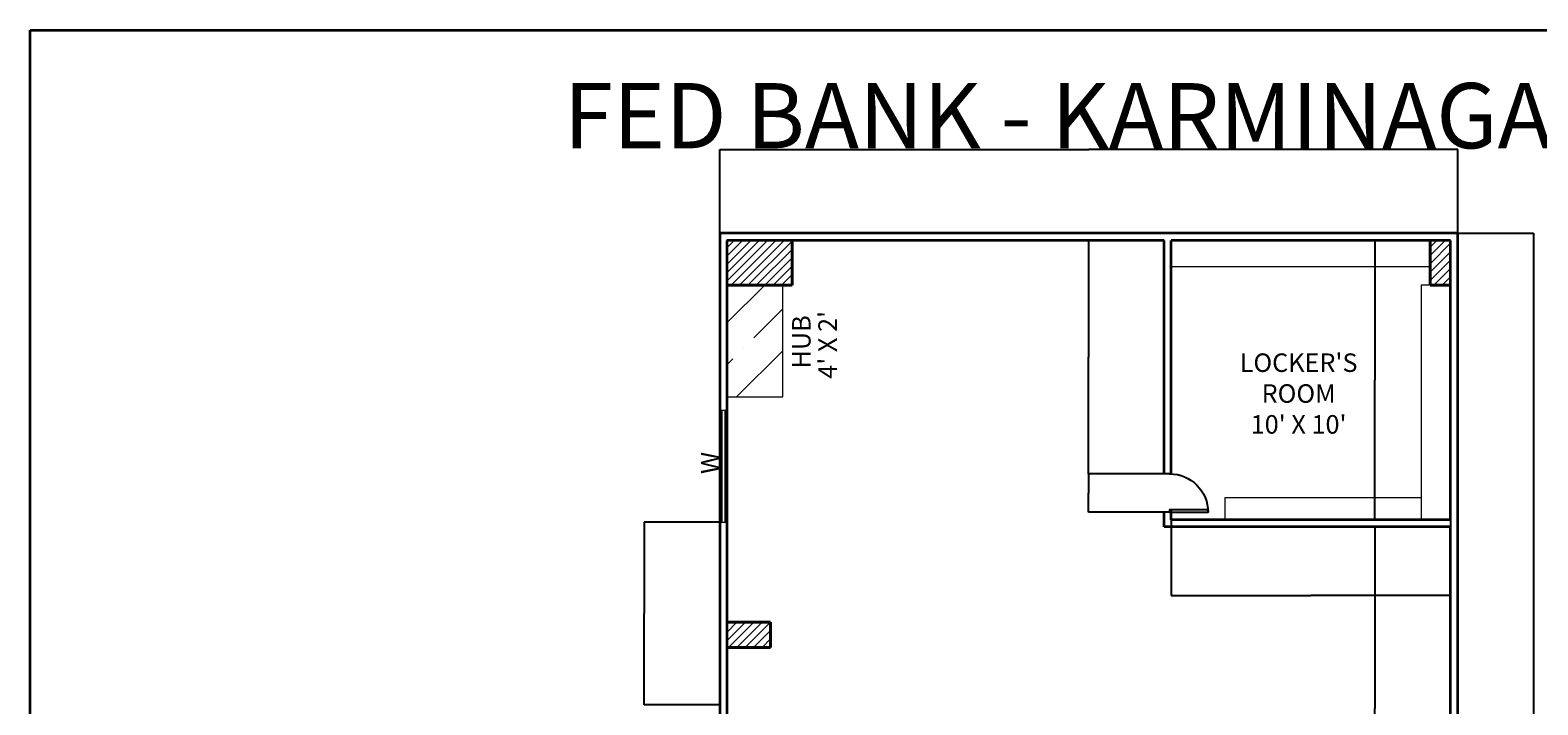
# Model space of a CAD drawing. Units: millimetres. Extents: x -5297 to 19051, y -14478 to 4427.
# Tile 3 of 4: x -5297 to 10888, y -2816 to 4427. Entities that reach past the tile are written whole.
import ezdxf

# ---------------------------------------------------------------- set-up
doc = ezdxf.new("R2010")
doc.units = ezdxf.units.MM
for name, color, linetype, lineweight in [('A-ANNO-DIMS', 2, 'Continuous', 18), ('A-ANNO-TEXT', 7, 'Continuous', 18), ('A-ANNO-TTLB', 7, 'Continuous', 35), ('A-AREA-IDEN', 7, 'Continuous', 25), ('A-COLS', 7, 'Continuous', 40), ('A-COLS-PATT', 252, 'Continuous', 13), ('A-DOOR', 3, 'Continuous', 25), ('A-EQPM', 8, 'Continuous', 20), ('A-EQPM-PATT', 252, 'Continuous', 13), ('A-FLOR-CASE', 9, 'Continuous', 20), ('A-GLAZ', 4, 'Continuous', 18), ('A-WALL', 7, 'Continuous', 35)]:
    doc.layers.add(name, color=color, linetype=linetype, lineweight=lineweight)
doc.styles.get("Standard").update_dxf_attribs({"font": 'arial.ttf'})
doc.dimstyles.get("Standard").update_dxf_attribs({"dimtxt": 0.18, "dimasz": 0.18, "dimexe": 0.18, "dimexo": 0.0625, "dimgap": 0.09, "dimtad": 0, "dimtih": 1, "dimtoh": 1, "dimdec": 4, "dimzin": 0, "dimdsep": 46, "dimtxsty": 'Standard', "dimcen": 0.09, "dimadec": 0, "dimazin": 0, "dimtfac": 1, "dimtdec": 4, "dimtofl": 0, "dimtmove": 0, "dimatfit": 3, "dimfxl": 1, "dimtolj": 1, "dimtzin": 0, "dimarcsym": 0})

# ---------------------------------------------------------------- blocks, each defined once
blk = doc.blocks.new('*U5')
for p, q in [((-700, 0), (-700, 99.99999999999996)), ((0, 0), (0, 99.99999999999999))]:
    blk.add_line(p, q)
blk.add_lwpolyline([(0, 0), (-1.137e-13, -700), (-43.75000000000011, -700), (-43.75, 1.42e-14)], close=True)
blk.add_arc((0, 0), 700, 180, 270)
blk = doc.blocks.new('WIN-1200')
for p, q in [((-4.547e-13, 1200.930645756219), (76.19999999999936, 1200.930645756219)), ((23.09999999999945, 1200.930645756219), (23.09999999999945, 0.9306457562195191)), ((53.09999999999945, 1200.930645756219), (53.09999999999945, 0.9306457562195191)), ((-4.547e-13, 0), (76.19999999999936, 0))]:
    blk.add_line(p, q)
blk = doc.blocks.new('*D20')
at = {"layer": 'A-ANNO-DIMS', "color": 0, "lineweight": -2, "transparency": 16777216}
for p, q in [((2105.501609, 2246.251823), (2105.501609, 3145.869928)), ((2105.681609, 3145.689928), (6066.344494402454, 3145.689928)), ((10027.721609, 3145.689928), (6067.058723597544, 3145.689928)), ((10027.901609, 2246.251823), (10027.901609, 3145.869928))]:
    blk.add_line(p, q, dxfattribs=at)
at = {"layer": 'A-ANNO-DIMS', "color": 0, "transparency": 16777216}
for points in [[(2105.681609, 3145.719928), (2105.681609, 3145.659928), (2105.501609, 3145.689928)], [(10027.721609, 3145.719928), (10027.721609, 3145.659928), (10027.901609, 3145.689928)]]:
    blk.add_solid(points, dxfattribs=at)
at = {"layer": 'Defpoints', "color": 0, "transparency": 16777216}
for p in [(10027.901609, 3145.689928), (2105.501609, 2246.189323), (10027.901609, 2246.189323)]:
    blk.add_point(p, dxfattribs=at)
at = {"layer": 'A-ANNO-DIMS', "color": 0, "transparency": 16777216, "insert": (6066.701608999999, 3145.689928), "char_height": 0.18, "attachment_point": 5}
blk.add_mtext('\\A1;7922', dxfattribs=at)
blk = doc.blocks.new('*D21')
at = {"layer": 'A-ANNO-DIMS', "color": 0, "lineweight": -2, "transparency": 16777216}
for p, q in [((10027.964109, 2246.189323000001), (10840.581609, 2246.189323000001)), ((10840.401609, 2246.009323000001), (10840.401609, -5417.56906597067)), ((10840.40160900001, -13081.511384), (10840.401609, -5417.932995029333)), ((10027.964109, -13081.691384), (10840.58160900001, -13081.691384))]:
    blk.add_line(p, q, dxfattribs=at)
at = {"layer": 'A-ANNO-DIMS', "color": 0, "transparency": 16777216}
for points in [[(10840.371609, 2246.009323000001), (10840.431609, 2246.009323000001), (10840.401609, 2246.189323000001)], [(10840.37160900001, -13081.511384), (10840.43160900001, -13081.511384), (10840.40160900001, -13081.691384)]]:
    blk.add_solid(points, dxfattribs=at)
at = {"layer": 'Defpoints', "color": 0, "transparency": 16777216}
for p in [(10027.901609, 2246.189323000001), (10027.901609, -13081.691384), (10840.40160900001, -13081.691384)]:
    blk.add_point(p, dxfattribs=at)
at = {"layer": 'A-ANNO-DIMS', "color": 0, "transparency": 16777216, "insert": (10840.401609, -5417.751030500004), "char_height": 0.18, "attachment_point": 5}
blk.add_mtext('\\A1;15328', dxfattribs=at)
blk = doc.blocks.new('*D24')
at = {"layer": 'A-ANNO-DIMS', "color": 0, "lineweight": -2, "transparency": 16777216}
for p, q in [((2105.439109000001, -854.7614690000004), (1292.821609, -854.7614690000006)), ((1293.001609, -854.9414690000006), (1293.001609000001, -1835.169301362211)), ((1293.001609000001, -2815.760940000001), (1293.001609000001, -1835.533107637791)), ((2105.439109000001, -2815.940940000001), (1292.821609000001, -2815.940940000001))]:
    blk.add_line(p, q, dxfattribs=at)
at = {"layer": 'A-ANNO-DIMS', "color": 0, "transparency": 16777216}
for points in [[(1292.971609, -854.9414690000006), (1293.031609, -854.9414690000006), (1293.001609, -854.7614690000006)], [(1292.971609000001, -2815.760940000001), (1293.031609000001, -2815.760940000001), (1293.001609000001, -2815.940940000001)]]:
    blk.add_solid(points, dxfattribs=at)
at = {"layer": 'Defpoints', "color": 0, "transparency": 16777216}
for p in [(1293.001609, -854.7614690000006), (2105.501609000001, -854.7614690000004), (2105.501609000001, -2815.940940000001)]:
    blk.add_point(p, dxfattribs=at)
at = {"layer": 'A-ANNO-DIMS', "color": 0, "transparency": 16777216, "insert": (1293.001609, -1835.351204500001), "char_height": 0.18, "attachment_point": 5}
blk.add_mtext('\\A1;1961', dxfattribs=at)
blk = doc.blocks.new('*D27')
at = {"layer": 'A-ANNO-DIMS', "color": 0, "lineweight": -2, "transparency": 16777216}
for p, q in [((9951.639109000005, -906.2106770000005), (9139.021609000007, -906.2106770000006)), ((9139.201609000007, -906.3906770000006), (9139.201609000007, -2854.82871247067)), ((9139.201609000009, -4803.630677000001), (9139.201609000007, -2855.192641529333)), ((9951.639109000005, -4803.810677000002), (9139.021609000009, -4803.810677000002))]:
    blk.add_line(p, q, dxfattribs=at)
at = {"layer": 'A-ANNO-DIMS', "color": 0, "transparency": 16777216}
for points in [[(9139.171609000006, -906.3906770000006), (9139.231609000008, -906.3906770000006), (9139.201609000007, -906.2106770000006)], [(9139.171609000008, -4803.630677000001), (9139.23160900001, -4803.630677000001), (9139.201609000009, -4803.810677000002)]]:
    blk.add_solid(points, dxfattribs=at)
at = {"layer": 'Defpoints', "color": 0, "transparency": 16777216}
for p in [(9139.201609000007, -906.2106770000006), (9951.701609000003, -906.2106770000005), (9951.701609000003, -4803.810677000002)]:
    blk.add_point(p, dxfattribs=at)
at = {"layer": 'A-ANNO-DIMS', "color": 0, "transparency": 16777216, "insert": (9139.201609000005, -2855.010677000003), "char_height": 0.18, "attachment_point": 5}
blk.add_mtext('\\A1;3897.6', dxfattribs=at)
blk = doc.blocks.new('*D28')
at = {"layer": 'A-ANNO-DIMS', "color": 0, "lineweight": -2, "transparency": 16777216}
for p, q in [((6951.701609, -830.073177), (6951.701609, -1642.690677)), ((9951.701609, -830.073177), (9951.701609, -1642.690677)), ((6951.881609, -1642.510677), (8451.34320518008, -1642.510677)), ((9951.521609, -1642.510677), (8452.060012819918, -1642.510677))]:
    blk.add_line(p, q, dxfattribs=at)
at = {"layer": 'A-ANNO-DIMS', "color": 0, "transparency": 16777216}
for points in [[(6951.881609, -1642.480677), (6951.881609, -1642.540677), (6951.701609, -1642.510677)], [(9951.521609, -1642.480677), (9951.521609, -1642.540677), (9951.701609, -1642.510677)]]:
    blk.add_solid(points, dxfattribs=at)
at = {"layer": 'Defpoints', "color": 0, "transparency": 16777216}
for p in [(6951.701609, -830.0106769999999), (9951.701609, -830.0106769999999), (6951.701609, -1642.510677)]:
    blk.add_point(p, dxfattribs=at)
at = {"layer": 'A-ANNO-DIMS', "color": 0, "transparency": 16777216, "insert": (8451.701609, -1642.510677), "char_height": 0.18, "attachment_point": 5}
blk.add_mtext('\\A1;3000', dxfattribs=at)
blk = doc.blocks.new('*D29')
at = {"layer": 'A-ANNO-DIMS', "color": 0, "lineweight": -2, "transparency": 16777216}
for p, q in [((9951.639109000005, 2169.989323000001), (9139.021609000007, 2169.989323000001)), ((9139.201609000007, 2169.809323), (9139.201609000007, 670.1712875293314)), ((9139.201609000007, -829.8306770000007), (9139.201609000007, 669.8073584706685)), ((9951.639109000005, -830.0106770000004), (9139.021609000007, -830.0106770000006))]:
    blk.add_line(p, q, dxfattribs=at)
at = {"layer": 'A-ANNO-DIMS', "color": 0, "transparency": 16777216}
for points in [[(9139.171609000006, 2169.809323), (9139.231609000008, 2169.809323), (9139.201609000007, 2169.989323000001)], [(9139.171609000006, -829.8306770000007), (9139.231609000008, -829.8306770000007), (9139.201609000007, -830.0106770000006)]]:
    blk.add_solid(points, dxfattribs=at)
at = {"layer": 'Defpoints', "color": 0, "transparency": 16777216}
for p in [(9139.201609000007, 2169.989323000001), (9951.701609000003, 2169.989323000001), (9951.701609000003, -830.0106770000004)]:
    blk.add_point(p, dxfattribs=at)
at = {"layer": 'A-ANNO-DIMS', "color": 0, "transparency": 16777216, "insert": (9139.201609000005, 669.9893229999973), "char_height": 0.18, "attachment_point": 5}
blk.add_mtext('\\A1;3000', dxfattribs=at)
blk = doc.blocks.new('*D33')
at = {"layer": 'A-ANNO-DIMS', "color": 0, "lineweight": -2, "transparency": 16777216}
for p, q in [((6875.439109000004, -335.8202160000001), (6062.821609000003, -335.8202160000002)), ((6063.001609000004, -336.0002160000003), (6063.001609000004, -542.3262389706689)), ((6063.001609000004, -749.0161910000003), (6063.001609000004, -542.6901680293317)), ((6875.439109000004, -749.1961910000002), (6062.821609000003, -749.1961910000003))]:
    blk.add_line(p, q, dxfattribs=at)
at = {"layer": 'A-ANNO-DIMS', "color": 0, "transparency": 16777216}
for points in [[(6062.971609000004, -336.0002160000003), (6063.031609000003, -336.0002160000003), (6063.001609000004, -335.8202160000002)], [(6062.971609000004, -749.0161910000003), (6063.031609000003, -749.0161910000003), (6063.001609000004, -749.1961910000003)]]:
    blk.add_solid(points, dxfattribs=at)
at = {"layer": 'Defpoints', "color": 0, "transparency": 16777216}
for p in [(6063.001609000004, -335.8202160000002), (6875.501609000004, -335.8202160000001), (6875.501609000004, -749.1961910000002)]:
    blk.add_point(p, dxfattribs=at)
at = {"layer": 'A-ANNO-DIMS', "color": 0, "transparency": 16777216, "insert": (6063.001609000003, -542.5082035000019), "char_height": 0.18, "attachment_point": 5}
blk.add_mtext('\\A1;413.4', dxfattribs=at)
blk = doc.blocks.new('*D34')
at = {"layer": 'A-ANNO-DIMS', "color": 0, "lineweight": -2, "transparency": 16777216}
for p, q in [((6875.439109000004, 2169.989323000001), (6062.821609000002, 2169.989323000001)), ((6063.001609000003, 2169.809323000001), (6063.001609000004, 917.2664566377902)), ((6063.001609000004, -335.6402160000002), (6063.001609000004, 916.9026503622104)), ((6875.439109000004, -335.8202160000001), (6062.821609000003, -335.8202160000002))]:
    blk.add_line(p, q, dxfattribs=at)
at = {"layer": 'A-ANNO-DIMS', "color": 0, "transparency": 16777216}
for points in [[(6062.971609000003, 2169.809323000001), (6063.031609000002, 2169.809323000001), (6063.001609000003, 2169.989323000001)], [(6062.971609000004, -335.6402160000002), (6063.031609000003, -335.6402160000002), (6063.001609000004, -335.8202160000002)]]:
    blk.add_solid(points, dxfattribs=at)
at = {"layer": 'Defpoints', "color": 0, "transparency": 16777216}
for p in [(6063.001609000003, 2169.989323000001), (6875.501609000004, 2169.989323000001), (6875.501609000004, -335.8202160000001)]:
    blk.add_point(p, dxfattribs=at)
at = {"layer": 'A-ANNO-DIMS', "color": 0, "transparency": 16777216, "insert": (6063.001609000003, 917.0845534999983), "char_height": 0.18, "attachment_point": 5}
blk.add_mtext('\\A1;2506', dxfattribs=at)

msp = doc.modelspace()

# ---------------------------------------------------------------- hatches: boundary and pattern name
at = {"layer": 'A-COLS-PATT'}
h = msp.add_hatch(dxfattribs=at)
h.set_pattern_fill('ANSI31', color=256, scale=20)
h.set_pattern_definition([(45, (0, 0), (-44.90128060534576, 44.90128060534576), [])])
h.paths.add_polyline_path([(2881.701609026896, 2169.989323322494), (2181.701609026895, 2169.989323322494), (2181.701609026895, 1689.989323322494), (2781.701609026896, 1689.989323322494), (2881.701609026895, 1689.989323322494)])
h.paths.add_polyline_path([(9951.701609026895, 2169.989323322494), (9731.701609026895, 2169.989323322494), (9731.701609026895, 1689.989323322494), (9951.701609026895, 1689.989323322494)])
h.paths.add_polyline_path([(2651.701609026896, -1930.010676677506), (2181.701609026895, -1930.010676677506), (2181.701609026895, -2200.010676677506), (2651.701609026896, -2200.010676677507)])
h.paths.add_polyline_path([(2661.701609026895, -5240.010676677506), (2181.701609026895, -5240.010676677506), (2181.701609026895, -5720.010676677507), (2661.701609026895, -5720.010676677507)])
h.paths.add_polyline_path([(2881.701609026896, -9690.010676677506), (2181.701609026895, -9690.010676677506), (2181.701609026895, -9960.010676677506), (2881.701609026896, -9960.010676677506)])
at = {"layer": 'A-EQPM-PATT'}
h = msp.add_hatch(dxfattribs=at)
h.set_pattern_fill('ANSI35', color=256, scale=100)
h.set_pattern_definition([(45, (0, 0), (-449.0128060534576, 449.0128060534576), []), (45, (449.013, 0), (-449.0128060534576, 449.0128060534576), [793.75, -158.75, 0, -158.75])])
h.paths.add_polyline_path([(2781.701609026896, 1689.989323322494), (2181.701609026895, 1689.989323322494), (2181.701609026895, 489.9893233224938), (2781.701609026896, 489.9893233224938)])

# ---------------------------------------------------------------- linework, layer by layer
at = {"layer": 'A-ANNO-TTLB'}
msp.add_lwpolyline([(-5297.042779185286, 4427.149582433107), (19050.70310178573, 4427.149582433107), (19050.70310178573, -14478.12049047724), (-5297.042779185286, -14478.12049047724)], close=True, dxfattribs=at)
at = {"layer": 'A-COLS'}
for p, q in [((2881.701609026896, 2169.989323322494), (2881.701609026895, 1689.989323322494)), ((9731.701609026895, 1689.989323322494), (9731.701609026895, 2169.989323322494)), ((2881.701609026896, 1689.989323322494), (2181.701609026895, 1689.989323322494)), ((9951.701609026895, 1689.989323322494), (9731.701609026895, 1689.989323322494)), ((2181.701609026895, -1930.010676677506), (2651.701609026896, -1930.010676677506)), ((2651.701609026896, -1930.010676677506), (2651.701609026896, -2200.010676677507)), ((2651.701609026896, -2200.010676677507), (2181.701609026895, -2200.010676677507))]:
    msp.add_line(p, q, dxfattribs=at)
at = {"layer": 'A-EQPM'}
for p, q in [((2181.701609026895, 1689.989323322494), (2181.701609026895, 489.9893233224941)), ((2781.701609026896, 1689.989323322494), (2181.701609026895, 1689.989323322494)), ((2181.701609026895, 1689.989323322494), (2181.701609026895, 489.9893233224938)), ((2781.701609026896, 1689.989323322494), (2181.701609026895, 1689.989323322494)), ((2781.701609026896, 489.9893233224938), (2781.701609026896, 1689.989323322494)), ((2181.701609026895, 489.9893233224938), (2781.701609026896, 489.9893233224938))]:
    msp.add_line(p, q, dxfattribs=at)
at = {"layer": 'A-FLOR-CASE'}
for p, q in [((6951.701609026894, 1889.895561774057), (9731.701609026895, 1889.895561774057)), ((9731.701609026895, 1689.989323322494), (9636.881912818588, 1689.989323322494)), ((9636.881912818588, 1689.989323322494), (9636.881912818588, -830.0106766775057)), ((9636.881912818588, -595.2302697078848), (7528.728212834917, -595.2302697078848)), ((7528.728212834917, -595.2302697078848), (7528.728212834917, -830.0106766775057)), ((9636.881912818588, -595.2302697078848), (9636.881912818588, -595.2302697078848))]:
    msp.add_line(p, q, dxfattribs=at)
at = {"layer": 'A-WALL'}
for p, q in [((2105.501609026896, 2246.189323322494), (2105.501609026896, -13080.86350256548)), ((10027.90160902689, 2246.189323322494), (2105.501609026896, 2246.189323322494)), ((2181.701609026895, 2169.989323322494), (2181.701609026895, -10503.8106766775)), ((6875.501609026895, 2169.989323322493), (2181.701609026895, 2169.989323322494)), ((6875.501609026897, -335.8202159030481), (6875.501609026895, 2169.989323322493)), ((9951.701609026895, 2169.989323322494), (6951.701609026897, 2169.989323322493)), ((6951.701609026897, -336.1759716969099), (6951.701609026895, 2169.989323322493)), ((9951.701609026895, -830.0106766775057), (9951.701609026895, 2169.989323322494)), ((10027.90160902689, -13081.69138398892), (10027.90160902689, 2246.189323322494)), ((6875.501609026895, -906.2106766775057), (6875.501609026897, -749.1961912871919)), ((6951.701609026897, -830.0106766775057), (6951.701609026897, -723.3601928256829)), ((9951.701609026895, -906.2106766775057), (6875.501609026897, -906.2106766775057)), ((9951.701609026895, -830.0106766775057), (6951.701609026897, -830.0106766775057)), ((9951.701609026897, -4803.810676677506), (9951.701609026893, -906.2106766775055))]:
    msp.add_line(p, q, dxfattribs=at)

# ---------------------------------------------------------------- block references
at = {"layer": 'A-DOOR', "xscale": -0.5905371076916341, "yscale": 0.5905371076916341, "zscale": 0.5905371076916341, "rotation": 90}
msp.add_blockref('*U5', (6934.55531979606, -749.1961912871919), dxfattribs=at)
at = {"layer": 'A-GLAZ'}
msp.add_blockref('WIN-1200', (2105.501609026896, -854.7614694249057), dxfattribs=at)

# ---------------------------------------------------------------- texts
at = {"layer": 'A-ANNO-TEXT', "char_height": 198.6149945558148, "attachment_point": 3, "rotation": 90.00000000000057}
for s, insert in [('\\pxqc;{\\fArial|b1|i0|c0|p34;HUB}', (2881.701609026896, 2481.126733761339)), ("\\pxqc;{\\fArial|b1|i0|c0|p34;4' X 2'}", (3163.925672626654, 2448.93839596951)), ('\\pxqc;{\\fArial|b1|i0|c0|p34;W}', (1903.499592053689, 1180.64946930963))]:
    msp.add_mtext_dynamic_manual_height_columns(s, width=2799.853245030821, gutter_width=413.7812386579476, heights=[0], dxfattribs=dict(at, insert=insert))
at = {"layer": 'A-ANNO-TTLB', "insert": (431.8611429029842, 3859.024494600358), "char_height": 700, "attachment_point": 1}
msp.add_mtext_dynamic_manual_height_columns('{\\fArial|b1|i0|c0|p34;FED BANK - KARMINAGAR}', width=12970.82879421404, gutter_width=826.634611161441, heights=[0], dxfattribs=at)
at = {"layer": 'A-AREA-IDEN', "insert": (9298.125493436668, 956.4986542072711), "char_height": 198.6149945558148, "attachment_point": 3}
msp.add_mtext_dynamic_manual_height_columns("\\pxqc;{\\fArial|b1|i0|c0|p34;LOCKER'S ROOM^J10' X 10'  }", width=1957.062248281983, gutter_width=413.7812386579476, heights=[0], dxfattribs=at)

# ---------------------------------------------------------------- dimensions: what is measured, and where the dimension line sits
at = {"layer": 'A-ANNO-DIMS'}
dim = msp.add_linear_dim(base=(10027.901609, 3145.689928), p1=(2105.501609, 2246.189323), p2=(10027.901609, 2246.189323), dimstyle='Standard', override={"dimdec": 0, "dimlfac": 1, "dimrnd": 0, "dimzin": 0, "dimdsep": 46, "dimlunit": 2}, dxfattribs=at)
dim.commit()
dim.dimension.update_dxf_attribs({"geometry": '*D20', "text_midpoint": (6066.701608999999, 3145.689928)})
for base, p1, p2, angle, override, picture, middle in [((6063.001609000003, 2169.989323000001), (6875.501609, -335.820216), (6875.501609, 2169.989323), 90.00000000000006, {"dimdec": 0, "dimlfac": 1, "dimrnd": 0, "dimzin": 0, "dimdsep": 46, "dimlunit": 2}, '*D34', (6063.001609000003, 917.0845534999983)), ((9139.201609000007, 2169.989323000001), (9951.701609, -830.0106769999999), (9951.701609, 2169.989323), 90, {"dimdec": 0, "dimlfac": 1, "dimrnd": 0, "dimzin": 0, "dimdsep": 46, "dimlunit": 2}, '*D29', (9139.201609000005, 669.9893229999973)), ((10840.40160900001, -13081.691384), (10027.901609, 2246.189323), (10027.901609, -13081.691384), 270, {"dimdec": 0, "dimlfac": 1, "dimrnd": 0, "dimzin": 0, "dimdsep": 46, "dimlunit": 2}, '*D21', (10840.401609, -5417.751030500004)), ((6063.001609000004, -335.8202160000002), (6875.501609, -749.196191), (6875.501609, -335.820216), 90, {"dimdec": 1, "dimlfac": 1, "dimrnd": 0, "dimzin": 0, "dimdsep": 46, "dimlunit": 2}, '*D33', (6063.001609000003, -542.5082035000019)), ((1293.001609, -854.7614690000006), (2105.501609, -2815.94094), (2105.501609, -854.7614690000001), 90, {"dimdec": 0, "dimlfac": 1, "dimrnd": 0, "dimzin": 0, "dimdsep": 46, "dimlunit": 2}, '*D24', (1293.001609, -1835.351204500001)), ((6951.701609, -1642.510677), (9951.701609, -830.0106769999999), (6951.701609, -830.0106769999999), 180, {"dimdec": 0, "dimlfac": 1, "dimrnd": 0, "dimzin": 0, "dimdsep": 46, "dimlunit": 2}, '*D28', (8451.701609, -1642.510677)), ((9139.201609000007, -906.2106770000006), (9951.701609, -4803.810677000001), (9951.701609, -906.2106769999999), 90.00000000000003, {"dimdec": 1, "dimlfac": 1, "dimrnd": 0, "dimzin": 0, "dimdsep": 46, "dimlunit": 2}, '*D27', (9139.201609000005, -2855.010677000003))]:
    dim = msp.add_linear_dim(base=base, p1=p1, p2=p2, angle=angle, dimstyle='Standard', override=override, dxfattribs=at)
    dim.commit()
    dim.dimension.update_dxf_attribs({"geometry": picture, "text_midpoint": middle})

doc.saveas('drawing.dxf')
